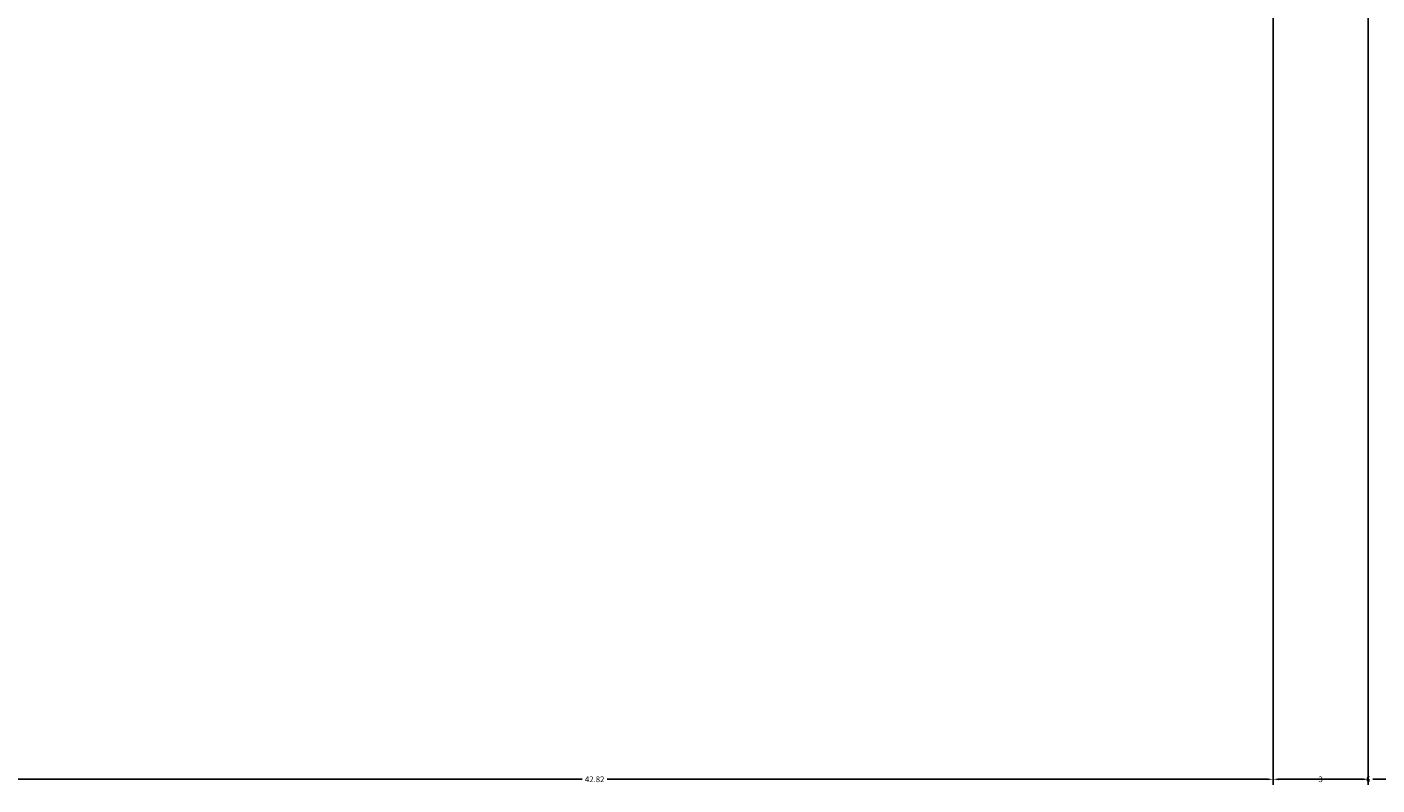
# Model space of a CAD drawing. Units: inches. Extents: x -1 to 292, y -3 to 199.
# Tile 2 of 52: x 25 to 68, y -3 to 21. Entities that reach past the tile are written whole.
import ezdxf

# ---------------------------------------------------------------- set-up
doc = ezdxf.new("R2010")
doc.units = ezdxf.units.IN
doc.header["$MEASUREMENT"] = 0
doc.layers.add('M-DIMS', color=2, linetype='Continuous', lineweight=18)
doc.styles.get("Standard").update_dxf_attribs({"font": 'arial.ttf'})
doc.dimstyles.get("Standard").update_dxf_attribs({"dimtxt": 0.18, "dimasz": 0.18, "dimexe": 0.18, "dimexo": 0.0625, "dimgap": 0.09, "dimtad": 0, "dimtih": 1, "dimtoh": 1, "dimdec": 4, "dimzin": 0, "dimdsep": 46, "dimtxsty": 'Standard', "dimcen": 0.09, "dimadec": 0, "dimazin": 0, "dimtfac": 1, "dimtdec": 4, "dimtofl": 0, "dimtmove": 0, "dimatfit": 3, "dimfxl": 1, "dimtolj": 1, "dimtzin": 0, "dimarcsym": 0})

# ---------------------------------------------------------------- blocks, each defined once
blk = doc.blocks.new('*D19')
at = {"layer": 'Defpoints', "color": 0, "transparency": 16777216}
for p in [(64.679, 51.267), (67.679, 51.267), (67.679, -2.71)]:
    blk.add_point(p, dxfattribs=at)
at = {"layer": 'M-DIMS', "color": 0, "lineweight": -2, "transparency": 16777216}
for p, q in [((64.679, 51.205), (64.679, -2.89)), ((67.679, 51.205), (67.679, -2.89)), ((64.859, -2.71), (66.03, -2.71)), ((67.499, -2.71), (66.328, -2.71))]:
    blk.add_line(p, q, dxfattribs=at)
at = {"layer": 'M-DIMS', "color": 0, "transparency": 16777216}
for points in [[(64.859, -2.68), (64.859, -2.74), (64.679, -2.71)], [(67.499, -2.68), (67.499, -2.74), (67.679, -2.71)]]:
    blk.add_solid(points, dxfattribs=at)
at = {"layer": 'M-DIMS', "color": 0, "transparency": 16777216, "insert": (66.179, -2.71), "char_height": 0.18, "attachment_point": 5}
blk.add_mtext('\\A1;3', dxfattribs=at)
blk = doc.blocks.new('*D20')
at = {"layer": 'Defpoints', "color": 0, "transparency": 16777216}
for p in [(64.679, 51.267), (70.679, 51.267), (70.679, -2.71)]:
    blk.add_point(p, dxfattribs=at)
at = {"layer": 'M-DIMS', "color": 0, "lineweight": -2, "transparency": 16777216}
for p, q in [((64.679, 51.205), (64.679, -2.89)), ((70.679, 51.205), (70.679, -2.89)), ((64.859, -2.71), (67.529, -2.71)), ((70.499, -2.71), (67.828, -2.71))]:
    blk.add_line(p, q, dxfattribs=at)
at = {"layer": 'M-DIMS', "color": 0, "transparency": 16777216}
for points in [[(64.859, -2.68), (64.859, -2.74), (64.679, -2.71)], [(70.499, -2.68), (70.499, -2.74), (70.679, -2.71)]]:
    blk.add_solid(points, dxfattribs=at)
at = {"layer": 'M-DIMS', "color": 0, "transparency": 16777216, "insert": (67.679, -2.71), "char_height": 0.18, "attachment_point": 5}
blk.add_mtext('\\A1;6', dxfattribs=at)
blk = doc.blocks.new('*D23')
at = {"layer": 'Defpoints', "color": 0, "transparency": 16777216}
for p in [(21.861, 54.582), (64.679, 51.267), (64.679, -2.71)]:
    blk.add_point(p, dxfattribs=at)
at = {"layer": 'M-DIMS', "color": 0, "lineweight": -2, "transparency": 16777216}
for p, q in [((21.861, 54.52), (21.861, -2.89)), ((64.679, 51.205), (64.679, -2.89)), ((22.041, -2.71), (42.874, -2.71)), ((64.499, -2.71), (43.666, -2.71))]:
    blk.add_line(p, q, dxfattribs=at)
at = {"layer": 'M-DIMS', "color": 0, "transparency": 16777216}
for points in [[(22.041, -2.68), (22.041, -2.74), (21.861, -2.71)], [(64.499, -2.68), (64.499, -2.74), (64.679, -2.71)]]:
    blk.add_solid(points, dxfattribs=at)
at = {"layer": 'M-DIMS', "color": 0, "transparency": 16777216, "insert": (43.27, -2.71), "char_height": 0.18, "attachment_point": 5}
blk.add_mtext('\\A1;42.82', dxfattribs=at)

msp = doc.modelspace()

# ---------------------------------------------------------------- dimensions: what is measured, and where the dimension line sits
at = {"layer": 'M-DIMS'}
for base, p1, p2, override, picture, middle in [((64.6788, -2.7104), (21.8612, 54.5821), (64.6788, 51.2672), {"dimdec": 2, "dimlfac": 1, "dimrnd": 0, "dimzin": 0, "dimdsep": 46, "dimlunit": 2}, '*D23', (43.27, -2.7104)), ((67.6788, -2.7104), (64.6788, 51.2672), (67.6788, 51.2672), {"dimdec": 0, "dimlfac": 1, "dimrnd": 0, "dimzin": 0, "dimdsep": 46, "dimlunit": 2}, '*D19', (66.1788, -2.7104)), ((70.6788, -2.7104), (64.6788, 51.2672), (70.6788, 51.2672), {"dimdec": 0, "dimlfac": 1, "dimrnd": 0, "dimzin": 0, "dimdsep": 46, "dimlunit": 2}, '*D20', (67.6788, -2.7104))]:
    dim = msp.add_linear_dim(base=base, p1=p1, p2=p2, dimstyle='Standard', override=override, dxfattribs=at)
    dim.commit()
    dim.dimension.update_dxf_attribs({"geometry": picture, "text_midpoint": middle})

doc.saveas('drawing.dxf')
